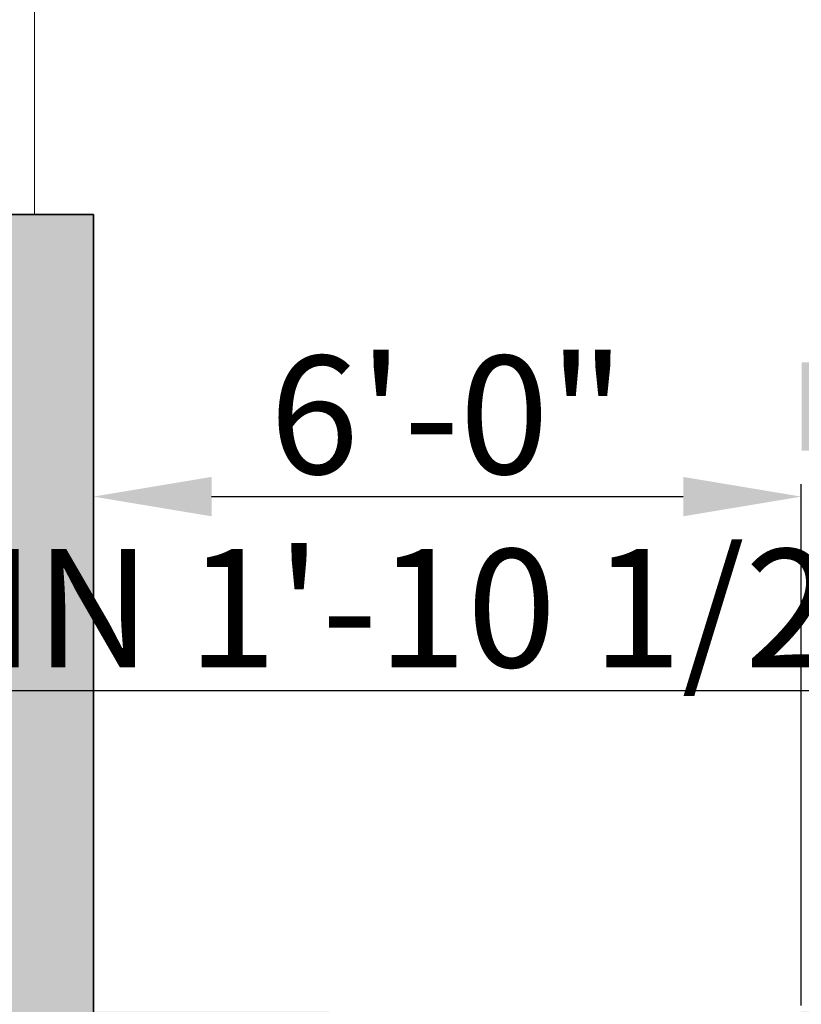
# Model space of a CAD drawing. Units: inches. Extents: x 2083 to 3317, y 1141 to 2115.
# Tile 114 of 256: x 2864 to 2944, y 1422 to 1522. Entities that reach past the tile are written whole.
import ezdxf

# ---------------------------------------------------------------- set-up
doc = ezdxf.new("R2010")
doc.units = ezdxf.units.IN
for name, color, linetype, lineweight in [('A-ANNO-DIMS', 2, 'Continuous', 18), ('A-GLAZ', 4, 'Continuous', 18), ('A-WALL', 7, 'Continuous', 35)]:
    doc.layers.add(name, color=color, linetype=linetype, lineweight=lineweight)
doc.layers.add('A-WALL-PATT', color=251, linetype='Continuous', lineweight=13, true_color=0x636466)
doc.styles.get("Standard").update_dxf_attribs({"font": 'arial.ttf'})
doc.dimstyles.new('ISO-25', dxfattribs={"dimtxt": 12, "dimasz": 12, "dimexe": 1.25, "dimexo": 0.625, "dimtad": 1, "dimlunit": 3, "dimtxsty": 'Standard', "dimcen": 2.5, "dimadec": 0, "dimazin": 0, "dimtfac": 1, "dimtmove": 0, "dimatfit": 3, "dimfxl": 1, "dimarcsym": 0})

# ---------------------------------------------------------------- blocks, each defined once
blk = doc.blocks.new('*D18')
at = {"layer": 'A-ANNO-DIMS', "color": 0, "lineweight": -2, "transparency": 16777216}
for p, q in [((3018.48, 1456.16), (3018.48, 1452.14)), ((3041.07, 1456.16), (3041.07, 1452.14)), ((3006.48, 1453.39), (2828.36, 1453.39)), ((3041.07, 1453.39), (3018.48, 1453.39)), ((3053.07, 1453.39), (3065.07, 1453.39))]:
    blk.add_line(p, q, dxfattribs=at)
at = {"layer": 'A-ANNO-DIMS', "color": 0, "transparency": 16777216}
for points in [[(3006.48, 1455.39), (3006.48, 1451.39), (3018.48, 1453.39)], [(3053.07, 1455.39), (3053.07, 1451.39), (3041.07, 1453.39)]]:
    blk.add_solid(points, dxfattribs=at)
at = {"layer": 'Defpoints', "color": 0, "transparency": 16777216}
for p in [(3018.48, 1456.78), (3041.07, 1456.78), (3018.48, 1453.39)]:
    blk.add_point(p, dxfattribs=at)
at = {"layer": 'A-ANNO-DIMS', "color": 0, "transparency": 16777216, "insert": (2911.42, 1460.22), "char_height": 12, "attachment_point": 5}
blk.add_mtext('BASIN 1\'-10 1/2" TYP.', dxfattribs=at)
blk = doc.blocks.new('*D48')
at = {"layer": 'A-ANNO-DIMS', "color": 0, "lineweight": -2, "transparency": 16777216}
for p, q in [((2871.96, 1421.39), (2871.96, 1474.36)), ((2943.91, 1421.39), (2943.91, 1474.36)), ((2883.96, 1473.11), (2931.91, 1473.11))]:
    blk.add_line(p, q, dxfattribs=at)
at = {"layer": 'A-ANNO-DIMS', "color": 0, "transparency": 16777216}
for points in [[(2883.96, 1475.11), (2883.96, 1471.11), (2871.96, 1473.11)], [(2931.91, 1475.11), (2931.91, 1471.11), (2943.91, 1473.11)]]:
    blk.add_solid(points, dxfattribs=at)
at = {"layer": 'Defpoints', "color": 0, "transparency": 16777216}
for p in [(2943.91, 1473.11), (2871.96, 1420.76), (2943.91, 1420.76)]:
    blk.add_point(p, dxfattribs=at)
at = {"layer": 'A-ANNO-DIMS', "color": 0, "transparency": 16777216, "insert": (2907.93, 1479.86), "char_height": 12, "attachment_point": 5}
blk.add_mtext('6\'-0"', dxfattribs=at)
blk = doc.blocks.new('*D57')
at = {"layer": 'A-ANNO-DIMS', "color": 0, "lineweight": -2, "transparency": 16777216}
for p, q in [((2871.33, 1621.76), (2818.36, 1621.76)), ((2819.61, 1513.76), (2819.61, 1609.76)), ((2871.33, 1501.76), (2818.36, 1501.76))]:
    blk.add_line(p, q, dxfattribs=at)
at = {"layer": 'A-ANNO-DIMS', "color": 0, "transparency": 16777216}
for points in [[(2817.61, 1609.76), (2821.61, 1609.76), (2819.61, 1621.76)], [(2817.61, 1513.76), (2821.61, 1513.76), (2819.61, 1501.76)]]:
    blk.add_solid(points, dxfattribs=at)
at = {"layer": 'Defpoints', "color": 0, "transparency": 16777216}
for p in [(2819.61, 1621.76), (2871.96, 1621.76), (2871.96, 1501.76)]:
    blk.add_point(p, dxfattribs=at)
at = {"layer": 'A-ANNO-DIMS', "color": 0, "transparency": 16777216, "insert": (2812.86, 1561.76), "char_height": 12, "attachment_point": 5, "rotation": 90}
blk.add_mtext('10\'-0"', dxfattribs=at)

msp = doc.modelspace()

# ---------------------------------------------------------------- hatches: boundary and pattern name
at = {"layer": 'A-WALL-PATT'}
h = msp.add_hatch(color=256, dxfattribs=at)
h.dxf.hatch_style = 1
h.paths.add_polyline_path([(3126.96, 2020.761), (2748.96, 2020.761), (2604.96, 2020.761), (2226.96, 2020.761), (2226.96, 1702.761), (2466.96, 1702.761), (2466.96, 1582.761), (2418.96, 1582.761), (2418.96, 1477.761), (2226.96, 1477.761), (2226.96, 1263.261), (2544.96, 1263.261), (2544.96, 1411.761), (2604.96, 1411.761), (2685.96, 1411.761), (2685.96, 1420.761), (2604.96, 1420.761), (2604.96, 1573.761), (2604.96, 1702.761), (2604.96, 2011.761), (2748.96, 2011.761), (2748.96, 1702.761), (2862.96, 1702.761), (2862.96, 1621.761), (2871.96, 1621.761), (2871.96, 1702.761), (2883.96, 1702.761), (2883.96, 1706.939, -0.0264593), (2883.96, 1711.761), (2757.96, 1711.761), (2757.96, 1807.761), (2787.96, 1807.761), (2787.96, 1812.261), (2757.96, 1812.261), (2757.96, 2011.761), (2877.96, 2011.761), (2877.96, 1812.261), (2847.96, 1812.261), (2847.96, 1807.761), (2889.836, 1807.761), (2889.836, 1812.261), (2882.46, 1812.261), (2882.46, 2011.761), (3117.96, 2011.761), (3117.96, 1812.261), (2937.836, 1812.261), (2937.836, 1807.761), (2995.71, 1807.761), (2995.71, 1796.118), (3000.21, 1796.118), (3000.21, 1807.761), (3117.96, 1807.761), (3117.96, 1711.761), (3000.21, 1711.761), (3000.21, 1760.118), (2998.573, 1760.118, -0.020711), (2995.71, 1760.118), (2995.71, 1711.761), (2931.96, 1711.761), (2931.96, 1702.761), (3126.96, 1702.761)])
h.paths.add_polyline_path([(2471.46, 2011.761), (2471.46, 1810.011), (2462.717, 1810.011), (2462.717, 1805.511), (2505.96, 1805.511), (2505.96, 1810.011), (2475.96, 1810.011), (2475.96, 2011.761), (2595.96, 2011.761), (2595.96, 1810.011), (2565.96, 1810.011), (2565.96, 1805.511), (2595.96, 1805.511), (2595.96, 1711.761), (2235.96, 1711.761), (2235.96, 1805.511), (2353.71, 1805.511), (2353.71, 1796.054), (2358.21, 1796.054), (2358.21, 1805.511), (2414.717, 1805.511), (2414.717, 1810.011), (2235.96, 1810.011), (2235.96, 2011.761)], flags=16)
h.paths.add_polyline_path([(2270.205, 1994.61), (2270.205, 1970.61), (2246.205, 1970.61), (2246.205, 1994.61)], flags=0)
edge = h.paths.add_edge_path(flags=0)
edge.add_ellipse((2332.027, 1899.798), major_axis=(-3.043, 3.043), ratio=0.1682525, start_angle=-161.33217, end_angle=-156.30711, ccw=False)
edge.add_ellipse((2333.082, 1898.744), major_axis=(-1.055, 1.055), ratio=0.4535321, start_angle=-123.37102, end_angle=-94.15911)
edge = h.paths.add_edge_path(flags=0)
edge.add_ellipse((2332.027, 1968.876), major_axis=(3.043, 3.043), ratio=0.1682525, start_angle=18.66783, end_angle=23.69289)
edge.add_spline(control_points=[(2332.926, 1970.691), (2332.227, 1970.336), (2330.894, 1969.659), (2328.413, 1970.932), (2327.204, 1967.749), (2324.71, 1969.956), (2322.533, 1967.012), (2320.013, 1971.296), (2317.68, 1968.158), (2316.041, 1967.102), (2315.427, 1966.81)], knot_values=[0, 0, 0, 0, 2.2670587, 4.3245589, 6.6855835, 8.8786411, 11.121502, 14.300359, 17.7552837, 19.732645, 19.732645, 19.732645, 19.732645], degree=3, periodic=0)
edge.add_ellipse((2332.027, 1968.876), major_axis=(3.043, 3.043), ratio=0.1682525, start_angle=18.66783, end_angle=23.69289, ccw=False)
edge.add_ellipse((2333.082, 1969.931), major_axis=(1.055, 1.055), ratio=0.4535321, start_angle=56.62898, end_angle=85.84089, ccw=False)
edge = h.paths.add_edge_path(flags=0)
edge.add_spline(control_points=[(2296.428, 1967.988), (2293.628, 1965.336), (2287.704, 1959.727), (2299.744, 1949.996), (2294.533, 1935.669), (2290.573, 1920.604), (2293.394, 1909.974), (2296.185, 1904.967)], knot_values=[0.0991853, 0.0991853, 0.0991853, 0.0991853, 0.3453009, 0.6198217, 0.9826526, 1.3860932, 1.8105546, 1.8105546, 1.8105546, 1.8105546], degree=3, periodic=0)
edge.add_spline(control_points=[(2296.185, 1904.967), (2297.384, 1902.619), (2298.001, 1901.949), (2298.553, 1901.468)], knot_values=[0.0062457, 0.0062457, 0.0062457, 0.0062457, 0.0554759, 0.0554759, 0.0554759, 0.0554759], degree=3, periodic=0)
edge.add_spline(control_points=[(2298.553, 1901.468), (2297.259, 1900.923), (2295.225, 1900.232), (2293.06, 1900.614), (2292.101, 1900.788), (2292.09, 1900.791)], knot_values=[0.3128349, 0.3128349, 0.3128349, 0.3128349, 0.4017797, 0.4749867, 0.4759027, 0.4759027, 0.4759027, 0.4759027], degree=3, periodic=0)
edge.add_arc((2292.794, 1904.664), 3.937, 215.4209, 259.69818, ccw=False)
edge.add_spline(control_points=[(2289.585, 1902.382), (2289.477, 1902.535), (2289.368, 1902.688), (2289.261, 1902.841)], knot_values=[0.1028719, 0.1028719, 0.1028719, 0.1028719, 0.1168958, 0.1168958, 0.1168958, 0.1168958], degree=3, periodic=0)
edge.add_spline(control_points=[(2289.261, 1902.841), (2288.687, 1902.55), (2287.64, 1902.02), (2285.881, 1901.874), (2283.853, 1901.504), (2281.72, 1899.711), (2278.467, 1899.493), (2276.157, 1901.883), (2272.259, 1899.804), (2267.778, 1901.843), (2262.244, 1900.184), (2257.415, 1901.782), (2254.318, 1900.726), (2253.178, 1900.337)], knot_values=[0, 0, 0, 0, 1.9079767, 3.4771759, 5.261074, 7.9728515, 11.6802485, 13.7179214, 16.9395917, 22.789562, 27.5025027, 33.5952153, 37.1456181, 37.1456181, 37.1456181, 37.1456181], degree=3, periodic=0)
edge.add_line((2253.178, 1900.337), (2250.244, 1902.841))
edge.add_line((2250.244, 1902.841), (2250.244, 1965.833))
edge.add_line((2250.244, 1965.833), (2253.178, 1968.337))
edge.add_spline(control_points=[(2253.178, 1968.337), (2254.318, 1967.948), (2257.415, 1966.892), (2262.244, 1968.49), (2267.778, 1966.831), (2271.527, 1968.537), (2273.876, 1967.828), (2274.207, 1967.728)], knot_values=[0, 0, 0, 0, 0.0901802, 0.2449351, 0.3646438, 0.5132331, 0.5378548, 0.5378548, 0.5378548, 0.5378548], degree=3, periodic=0)
edge.add_arc((2274.353, 1963.793), 3.937, 72.05113, 92.12795, ccw=False)
edge.add_arc((2281.297, 1985.23), 18.596, 252.05113, 288.56572)
edge.add_arc((2292.317, 1956.029), 12.646, 71.02679, 113.77822, ccw=False)
edge = h.paths.add_edge_path(flags=0)
edge.add_spline(control_points=[(2274.899, 1951.856), (2275.066, 1951.617), (2275.233, 1951.377), (2275.398, 1951.136)], knot_values=[1.4099157, 1.4099157, 1.4099157, 1.4099157, 1.4315903, 1.4315903, 1.4315903, 1.4315903], degree=3, periodic=0)
edge.add_spline(control_points=[(2275.398, 1951.136), (2275.792, 1950.562), (2276.179, 1949.984), (2276.546, 1949.397)], knot_values=[1.3582378, 1.3582378, 1.3582378, 1.3582378, 1.4099157, 1.4099157, 1.4099157, 1.4099157], degree=3, periodic=0)
edge.add_line((2276.546, 1949.397), (2277.437, 1947.862))
edge.add_spline(control_points=[(2277.437, 1947.862), (2276.304, 1945.673), (2274.64, 1942.427), (2274.632, 1938.094), (2272.799, 1930.852), (2274.356, 1943.897), (2275.948, 1947.923), (2276.546, 1949.397)], knot_values=[0.0056315, 0.0056315, 0.0056315, 0.0056315, 0.1860139, 0.2660015, 0.3570872, 0.5963902, 0.7397317, 0.7397317, 0.7397317, 0.7397317], degree=3, periodic=0)
edge.add_spline(control_points=[(2276.546, 1949.397), (2276.179, 1949.984), (2275.792, 1950.562), (2275.398, 1951.136)], knot_values=[1.3582378, 1.3582378, 1.3582378, 1.3582378, 1.4099157, 1.4099157, 1.4099157, 1.4099157], degree=3, periodic=0)
edge.add_spline(control_points=[(2275.398, 1951.136), (2274.943, 1950.08), (2274.208, 1948.025), (2273.935, 1944.851), (2272.469, 1937.627), (2273.466, 1945.696), (2274.701, 1951.059), (2274.899, 1951.856)], knot_values=[0.1043639, 0.1043639, 0.1043639, 0.1043639, 0.1896363, 0.2696239, 0.3607096, 0.6000126, 0.6446217, 0.6446217, 0.6446217, 0.6446217], degree=3, periodic=0)
h.paths.add_polyline_path([(2269.168, 1963.128, -0.3575267), (2268.171, 1960.976, -0.0925607), (2268.171, 1939.436, -0.3575267), (2269.168, 1937.285, -0.3575267), (2267.016, 1938.282, -0.1647847), (2254.686, 1938.282, -0.3575267), (2252.534, 1937.285, -0.3575267), (2253.531, 1939.436, -0.0925607), (2253.531, 1960.976, -0.3575267), (2252.534, 1963.128, -0.3575267), (2254.686, 1962.131, -0.1647847), (2267.016, 1962.131, -0.3575267)], flags=0)
h.paths.add_polyline_path([(2248.874, 1967.802), (2248.874, 1957.028), (2249.458, 1957.028), (2249.458, 1911.647), (2248.874, 1911.647), (2248.874, 1900.873), (2246.512, 1900.873, 0.1973271), (2244.15, 1902.457), (2244.15, 1966.218, 0.1973271), (2246.512, 1967.802)], flags=0)
h.paths.add_polyline_path([(2269.168, 1931.389, -0.3575267), (2268.171, 1929.238, -0.0925607), (2268.171, 1907.698, -0.3575267), (2269.168, 1905.547, -0.3575267), (2267.016, 1906.544, -0.1647847), (2254.686, 1906.544, -0.3575267), (2252.534, 1905.547, -0.3575267), (2253.531, 1907.698, -0.0925607), (2253.531, 1929.238, -0.3575267), (2252.534, 1931.389, -0.3575267), (2254.686, 1930.392, -0.1647847), (2267.016, 1930.392, -0.3575267)], flags=0)
edge = h.paths.add_edge_path(flags=0)
edge.add_spline(control_points=[(2276.197, 1906.724), (2276.168, 1909.029), (2276.114, 1913.372), (2270.598, 1924.925), (2273.905, 1919.013), (2275.922, 1916.262), (2275.475, 1912.402), (2277.258, 1910.381), (2276.696, 1908.225), (2276.646, 1906.813), (2276.618, 1906.008)], knot_values=[0, 0, 0, 0, 8.6102597, 16.2212739, 18.8430575, 23.8048978, 27.4408283, 29.3561016, 31.2034776, 33.6506866, 33.6506866, 33.6506866, 33.6506866], degree=3, periodic=0)
edge.add_spline(control_points=[(2276.618, 1906.008), (2276.623, 1905.624), (2276.498, 1904.629), (2275.442, 1903.855), (2274.937, 1903.08), (2274.859, 1902.841)], knot_values=[0.1564884, 0.1564884, 0.1564884, 0.1564884, 0.1843975, 0.2313765, 0.2505985, 0.2505985, 0.2505985, 0.2505985], degree=3, periodic=0)
edge.add_line((2274.859, 1902.841), (2276.506, 1902.841))
edge.add_spline(control_points=[(2276.506, 1902.841), (2276.788, 1903.085), (2277.665, 1904.125), (2278.25, 1904.341), (2277.654, 1908.527), (2278.156, 1906.228), (2278.1, 1905.286), (2278.847, 1904.069), (2277.857, 1903.415), (2277.874, 1902.991), (2277.904, 1902.841)], knot_values=[0.0595743, 0.0595743, 0.0595743, 0.0595743, 0.0807529, 0.1037415, 0.1697201, 0.1760361, 0.2071372, 0.2404744, 0.2623409, 0.2736605, 0.2736605, 0.2736605, 0.2736605], degree=3, periodic=0)
edge.add_line((2277.904, 1902.841), (2280.03, 1902.841))
edge.add_spline(control_points=[(2280.03, 1902.841), (2279.888, 1903.088), (2279.499, 1903.982), (2280.152, 1905.939), (2278.104, 1909.658), (2279.762, 1907.185), (2280.328, 1904.875), (2280.485, 1903.49), (2281.463, 1903.249), (2281.758, 1902.936), (2281.834, 1902.841)], knot_values=[0.013856, 0.013856, 0.013856, 0.013856, 0.0348738, 0.0888667, 0.1078792, 0.1267378, 0.158714, 0.1937575, 0.2174868, 0.2267221, 0.2267221, 0.2267221, 0.2267221], degree=3, periodic=0)
edge.add_spline(control_points=[(2281.834, 1902.841), (2281.788, 1902.827), (2281.647, 1902.783), (2281.396, 1902.859), (2281.088, 1902.985), (2280.721, 1903.061), (2280.333, 1903.026), (2280.125, 1902.899), (2280.03, 1902.841)], knot_values=[0, 0, 0, 0, 0.1441304, 0.435517, 0.7492759, 1.1530457, 1.5483707, 1.878348, 1.878348, 1.878348, 1.878348], degree=3, periodic=0)
edge.add_line((2280.03, 1902.841), (2277.904, 1902.841))
edge.add_spline(control_points=[(2277.904, 1902.841), (2277.893, 1902.796), (2277.865, 1902.68), (2277.607, 1902.687), (2277.274, 1902.801), (2276.838, 1902.62), (2276.584, 1902.789), (2276.506, 1902.841)], knot_values=[0, 0, 0, 0, 0.1271885, 0.3261988, 0.6280094, 1.2435704, 1.5153306, 1.5153306, 1.5153306, 1.5153306], degree=3, periodic=0)
edge.add_line((2276.506, 1902.841), (2274.859, 1902.841))
edge.add_spline(control_points=[(2274.859, 1902.841), (2274.814, 1902.899), (2274.725, 1903.013), (2274.493, 1903.119), (2274.244, 1902.961), (2273.937, 1903.185), (2273.614, 1902.983), (2273.408, 1902.883), (2273.322, 1902.841)], knot_values=[0, 0, 0, 0, 0.2184302, 0.4369566, 0.6879766, 0.9903786, 1.3983955, 1.6918498, 1.6918498, 1.6918498, 1.6918498], degree=3, periodic=0)
edge.add_spline(control_points=[(2273.322, 1902.841), (2273.617, 1903.446), (2274.274, 1904.538), (2276.027, 1904.574), (2276.207, 1906.584), (2276.197, 1906.724)], knot_values=[0.0122268, 0.0122268, 0.0122268, 0.0122268, 0.0594721, 0.1062177, 0.134458, 0.134458, 0.134458, 0.134458], degree=3, periodic=0)
h.paths.add_polyline_path([(2270.776, 1897.79), (2270.776, 1873.79), (2246.776, 1873.79), (2246.776, 1897.79)], flags=0)
h.paths.add_polyline_path([(2353.71, 1760.005), (2353.71, 1760.054), (2358.21, 1760.054, -0.033729)], flags=0)
h.paths.add_polyline_path([(2321.819, 1737.529), (2341.995, 1737.529, -0.4142136), (2343.203, 1736.321), (2343.203, 1721.021, -0.4142136), (2341.995, 1719.813), (2321.819, 1719.813, -0.4142136), (2320.611, 1721.021), (2320.611, 1736.321, -0.4142136)], flags=0)
h.paths.add_polyline_path([(2324.235, 1736.321), (2339.579, 1736.321, -0.4142136), (2341.995, 1733.905), (2341.995, 1725.45, -0.4142136), (2339.579, 1723.034), (2333.681, 1723.034), (2333.845, 1722.045, -0.8706461), (2335.425, 1721.826, -0.767327), (2333.923, 1721.423), (2331.291, 1721.423, -0.767327), (2329.788, 1721.826, -0.8706461), (2331.368, 1722.045), (2331.533, 1723.034), (2324.235, 1723.034, -0.4142136), (2321.819, 1725.45), (2321.819, 1733.905, -0.4142136)], flags=0)
h.paths.add_polyline_path([(2570.484, 1928.615), (2589.684, 1928.615), (2590.169, 1928.615), (2590.169, 1904.993), (2570.484, 1904.993)], flags=0)
h.paths.add_polyline_path([(2574.447, 1927.264, -1), (2572.829, 1927.264, -1)], flags=0)
h.paths.add_polyline_path([(2573.09, 1926.941), (2573.925, 1927.776), (2574.148, 1927.553), (2573.313, 1926.718)], flags=0)
h.paths.add_polyline_path([(2578.779, 1919.73, -1), (2571.592, 1919.73, -1)], flags=0)
h.paths.add_polyline_path([(2578.385, 1919.73, -1), (2571.985, 1919.73, -1)], flags=0)
h.paths.add_polyline_path([(2331.596, 1729.476, -1), (2333.618, 1729.476, -1)], flags=0)
h.paths.add_polyline_path([(2578.034, 1927.264, -1), (2576.416, 1927.264, -1)], flags=0)
h.paths.add_polyline_path([(2576.689, 1927.531), (2576.912, 1927.754), (2577.747, 1926.919), (2577.524, 1926.696)], flags=0)
h.paths.add_polyline_path([(2578.139, 1909.86, -1), (2572.232, 1909.86, -1)], flags=0)
h.paths.add_polyline_path([(2577.745, 1909.86, -1), (2572.625, 1909.86, -1)], flags=0)
h.paths.add_polyline_path([(2583.798, 1927.264, -1), (2582.179, 1927.264, -1)], flags=0)
h.paths.add_polyline_path([(2582.719, 1927.754), (2583.554, 1926.919), (2583.331, 1926.696), (2582.496, 1927.531)], flags=0)
h.paths.add_polyline_path([(2582.496, 1927.531), (2582.719, 1927.754), (2583.554, 1926.919), (2583.331, 1926.696)], flags=0)
h.paths.add_polyline_path([(2587.739, 1920.53, -1), (2581.832, 1920.53, -1)], flags=0)
h.paths.add_polyline_path([(2587.345, 1920.53, -1), (2582.225, 1920.53, -1)], flags=0)
h.paths.add_polyline_path([(2587.385, 1927.264, -1), (2585.766, 1927.264, -1)], flags=0)
h.paths.add_polyline_path([(2586.082, 1926.98), (2586.917, 1927.815), (2587.14, 1927.593), (2586.305, 1926.758)], flags=0)
h.paths.add_polyline_path([(2588.379, 1910.66, -1), (2581.192, 1910.66, -1)], flags=0)
h.paths.add_polyline_path([(2587.985, 1910.66, -1), (2581.585, 1910.66, -1)], flags=0)
h.paths.add_polyline_path([(2417.168, 1729.478), (2437.344, 1729.478, -0.4142136), (2438.552, 1728.27), (2438.552, 1712.969, -0.4142136), (2437.344, 1711.761), (2417.168, 1711.761, -0.4142136), (2415.96, 1712.969), (2415.96, 1728.27, -0.4142136)], flags=0)
h.paths.add_polyline_path([(2419.584, 1728.27), (2434.928, 1728.27, -0.4142136), (2437.344, 1725.854), (2437.344, 1717.398, -0.4142136), (2434.928, 1714.983), (2429.029, 1714.983), (2429.194, 1713.994, -0.8706461), (2430.774, 1713.775, -0.767327), (2429.271, 1713.372), (2426.64, 1713.372, -0.767327), (2425.137, 1713.775, -0.8706461), (2426.717, 1713.994), (2426.882, 1714.983), (2419.584, 1714.983, -0.4142136), (2417.168, 1717.398), (2417.168, 1725.854, -0.4142136)], flags=0)
h.paths.add_polyline_path([(2419.584, 1728.27), (2434.928, 1728.27, -0.4142136), (2437.344, 1725.854), (2437.344, 1717.398, -0.4142136), (2434.928, 1714.983), (2429.029, 1714.983), (2428.358, 1719.009), (2427.553, 1719.009), (2426.882, 1714.983), (2419.584, 1714.983, -0.4142136), (2417.168, 1717.398), (2417.168, 1725.854, -0.4142136)], flags=0)
h.paths.add_polyline_path([(2426.944, 1721.425, -1), (2428.967, 1721.425, -1)], flags=0)
h.paths.add_polyline_path([(2475.96, 1702.761), (2595.96, 1702.761), (2595.96, 1582.761), (2475.96, 1582.761)], flags=16)
h.paths.add_polyline_path([(2427.96, 1573.761), (2595.96, 1573.761), (2595.96, 1468.761), (2595.96, 1420.761), (2384.46, 1420.761), (2384.46, 1468.761), (2427.96, 1468.761)], flags=16)
h.paths.add_polyline_path([(2379.96, 1468.761), (2379.96, 1420.761), (2235.96, 1420.761), (2235.96, 1468.761)], flags=16)
h.paths.add_polyline_path([(2317.816, 1466.696), (2337.992, 1466.696, -0.4142136), (2339.2, 1465.488), (2339.2, 1450.187, -0.4142136), (2337.992, 1448.979), (2317.816, 1448.979, -0.4142136), (2316.608, 1450.187), (2316.608, 1465.488, -0.4142136)], flags=0)
h.paths.add_polyline_path([(2320.232, 1465.488), (2335.576, 1465.488, -0.4142136), (2337.992, 1463.072), (2337.992, 1454.616, -0.4142136), (2335.576, 1452.2), (2329.677, 1452.2), (2329.842, 1451.212, -0.8706461), (2331.422, 1450.992, -0.767327), (2329.92, 1450.59), (2327.288, 1450.59, -0.767327), (2325.785, 1450.992, -0.8706461), (2327.365, 1451.212), (2327.53, 1452.2), (2320.232, 1452.2, -0.4142136), (2317.816, 1454.616), (2317.816, 1463.072, -0.4142136)], flags=0)
h.paths.add_polyline_path([(2320.232, 1465.488), (2335.576, 1465.488, -0.4142136), (2337.992, 1463.072), (2337.992, 1454.616, -0.4142136), (2335.576, 1452.2), (2329.677, 1452.2), (2329.006, 1456.227), (2328.201, 1456.227), (2327.53, 1452.2), (2320.232, 1452.2, -0.4142136), (2317.816, 1454.616), (2317.816, 1463.072, -0.4142136)], flags=0)
h.paths.add_polyline_path([(2327.593, 1458.643, -1), (2329.615, 1458.643, -1)], flags=0)
h.paths.add_polyline_path([(2244.412, 1433.34), (2241.921, 1433.34, -0.4142136), (2240.018, 1435.244), (2240.018, 1440.953, -0.4142105), (2241.921, 1442.856), (2244.412, 1442.856, -1.9764724)], flags=0)
h.paths.add_polyline_path([(2245.357, 1434.398, -0.4142136), (2245.357, 1441.799, -2.1440985)], flags=0)
h.paths.add_polyline_path([(2535.96, 1416.261), (2535.96, 1272.261), (2235.96, 1272.261), (2235.96, 1416.261)], flags=16)
h.paths.add_polyline_path([(2260.12, 1384.293), (2260.12, 1362.039), (2237.865, 1362.039), (2237.865, 1384.293)], flags=0)
edge = h.paths.add_edge_path(flags=0)
edge.add_line((2318.252, 1362.093), (2318.146, 1362.001))
edge.add_ellipse((2317.445, 1360.431), major_axis=(2.822, 2.822), ratio=0.1682525, start_angle=18.66783, end_angle=20.94813, ccw=False)
edge.add_ellipse((2318.423, 1361.409), major_axis=(0.978, 0.978), ratio=0.4535321, start_angle=56.62898, end_angle=70.2262, ccw=False)
edge = h.paths.add_edge_path(flags=0)
edge.add_line((2319.107, 1295.571), (2319.015, 1295.677))
edge.add_ellipse((2317.445, 1296.378), major_axis=(-2.822, 2.822), ratio=0.1682525, start_angle=-161.33217, end_angle=-159.05187, ccw=False)
edge.add_ellipse((2318.423, 1295.4), major_axis=(-0.978, 0.978), ratio=0.4535321, start_angle=-123.37102, end_angle=-109.7738)
edge = h.paths.add_edge_path(flags=0)
edge.add_spline(control_points=[(2284.21, 1301.17), (2284.581, 1300.445), (2284.891, 1299.892), (2285.16, 1299.461)], knot_values=[0.0390658, 0.0390658, 0.0390658, 0.0390658, 0.0554759, 0.0554759, 0.0554759, 0.0554759], degree=3, periodic=0)
edge.add_line((2285.16, 1299.461), (2284.21, 1301.17))
edge = h.paths.add_edge_path(flags=0)
edge.add_line((2280.412, 1297.298), (2283.37, 1297.036))
edge.add_line((2283.37, 1297.036), (2286.406, 1297.926))
edge.add_spline(control_points=[(2286.406, 1297.926), (2285.305, 1297.463), (2284.345, 1297.129), (2283.37, 1297.036)], knot_values=[0.3943688, 0.3943688, 0.3943688, 0.3943688, 0.4759027, 0.4759027, 0.4759027, 0.4759027], degree=3, periodic=0)
edge.add_spline(control_points=[(2283.37, 1297.036), (2283.281, 1297.028), (2282.316, 1296.957), (2281.313, 1297.134), (2280.423, 1297.296), (2280.412, 1297.298)], knot_values=[0.3128349, 0.3128349, 0.3128349, 0.3128349, 0.3202458, 0.3934528, 0.3943688, 0.3943688, 0.3943688, 0.3943688], degree=3, periodic=0)
edge = h.paths.add_edge_path(flags=0)
edge.add_line((2284.436, 1359.607), (2280.446, 1355.328))
edge.add_line((2280.446, 1355.328), (2279.58, 1351.018))
edge.add_line((2279.58, 1351.018), (2282.413, 1346.58))
edge.add_spline(control_points=[(2282.413, 1346.58), (2283.153, 1345.589), (2284.253, 1344.029), (2284.801, 1342.387), (2284.935, 1341.806)], knot_values=[1.2400982, 1.2400982, 1.2400982, 1.2400982, 1.3328922, 1.3827123, 1.3827123, 1.3827123, 1.3827123], degree=3, periodic=0)
edge.add_spline(control_points=[(2284.935, 1341.806), (2285.319, 1340.141), (2285.233, 1338.409), (2284.91, 1336.654)], knot_values=[1.0974841, 1.0974841, 1.0974841, 1.0974841, 1.2400982, 1.2400982, 1.2400982, 1.2400982], degree=3, periodic=0)
edge.add_spline(control_points=[(2284.91, 1336.654), (2284.587, 1334.899), (2284.027, 1333.12), (2283.463, 1331.361)], knot_values=[0.9548699, 0.9548699, 0.9548699, 0.9548699, 1.0974841, 1.0974841, 1.0974841, 1.0974841], degree=3, periodic=0)
edge.add_line((2283.463, 1331.361), (2281.89, 1326.153))
edge.add_line((2281.89, 1326.153), (2280.756, 1321.056))
edge.add_line((2280.756, 1321.056), (2280.299, 1316.002))
edge.add_line((2280.299, 1316.002), (2280.716, 1310.95))
edge.add_line((2280.716, 1310.95), (2282.028, 1305.972))
edge.add_line((2282.028, 1305.972), (2284.21, 1301.17))
edge.add_spline(control_points=[(2284.21, 1301.17), (2283.341, 1302.73), (2282.612, 1304.336), (2282.028, 1305.972)], knot_values=[0.0991853, 0.0991853, 0.0991853, 0.0991853, 0.2417994, 0.2417994, 0.2417994, 0.2417994], degree=3, periodic=0)
edge.add_spline(control_points=[(2282.028, 1305.972), (2281.444, 1307.608), (2281.005, 1309.273), (2280.716, 1310.95)], knot_values=[0.2417994, 0.2417994, 0.2417994, 0.2417994, 0.3844135, 0.3844135, 0.3844135, 0.3844135], degree=3, periodic=0)
edge.add_spline(control_points=[(2280.716, 1310.95), (2280.433, 1312.588), (2280.289, 1314.277), (2280.299, 1315.962), (2280.299, 1316.002)], knot_values=[0.3844135, 0.3844135, 0.3844135, 0.3844135, 0.5236467, 0.5270276, 0.5270276, 0.5270276, 0.5270276], degree=3, periodic=0)
edge.add_spline(control_points=[(2280.299, 1316.002), (2280.312, 1317.687), (2280.478, 1319.368), (2280.756, 1321.056)], knot_values=[0.5270276, 0.5270276, 0.5270276, 0.5270276, 0.6696417, 0.6696417, 0.6696417, 0.6696417], degree=3, periodic=0)
edge.add_spline(control_points=[(2280.756, 1321.056), (2281.035, 1322.744), (2281.426, 1324.44), (2281.89, 1326.153)], knot_values=[0.6696417, 0.6696417, 0.6696417, 0.6696417, 0.8122558, 0.8122558, 0.8122558, 0.8122558], degree=3, periodic=0)
edge.add_spline(control_points=[(2281.89, 1326.153), (2282.264, 1327.533), (2282.788, 1329.262), (2283.353, 1331.018), (2283.463, 1331.361)], knot_values=[0.8122558, 0.8122558, 0.8122558, 0.8122558, 0.9270873, 0.9548699, 0.9548699, 0.9548699, 0.9548699], degree=3, periodic=0)
edge.add_line((2283.463, 1331.361), (2284.91, 1336.654))
edge.add_line((2284.91, 1336.654), (2284.935, 1341.806))
edge.add_line((2284.935, 1341.806), (2282.413, 1346.58))
edge.add_spline(control_points=[(2282.413, 1346.58), (2281.275, 1348.104), (2280.078, 1349.57), (2279.58, 1351.018)], knot_values=[1.3827123, 1.3827123, 1.3827123, 1.3827123, 1.5253264, 1.5253264, 1.5253264, 1.5253264], degree=3, periodic=0)
edge.add_spline(control_points=[(2279.58, 1351.018), (2279.443, 1351.415), (2279.136, 1352.857), (2279.735, 1354.29), (2280.446, 1355.328)], knot_values=[1.5253264, 1.5253264, 1.5253264, 1.5253264, 1.564439, 1.6679405, 1.6679405, 1.6679405, 1.6679405], degree=3, periodic=0)
edge.add_spline(control_points=[(2280.446, 1355.328), (2281.426, 1356.758), (2282.931, 1358.183), (2284.436, 1359.607)], knot_values=[1.6679405, 1.6679405, 1.6679405, 1.6679405, 1.8105546, 1.8105546, 1.8105546, 1.8105546], degree=3, periodic=0)
edge.add_arc((2280.623, 1348.518), 11.726, 71.02679, 113.77822)
edge.add_arc((2270.405, 1375.595), 17.244, 252.05113, 288.56572, ccw=False)
edge.add_arc((2263.966, 1355.718), 3.651, 72.05113, 92.12795)
edge.add_arc((2263.966, 1355.718), 3.651, 92.12795, 177.98513)
edge.add_spline(control_points=[(2260.318, 1355.846), (2260.26, 1354.221), (2260.551, 1350.187), (2262.999, 1346.766), (2264.473, 1344.649)], knot_values=[1.4315903, 1.4315903, 1.4315903, 1.4315903, 1.5641438, 1.7706953, 1.7706953, 1.7706953, 1.7706953], degree=3, periodic=0)
edge.add_line((2264.473, 1344.649), (2264.936, 1343.983))
edge.add_spline(control_points=[(2263.801, 1340.248), (2263.843, 1340.514), (2264.067, 1341.756), (2264.513, 1343.002), (2264.935, 1343.981)], knot_values=[0.5365702, 0.5365702, 0.5365702, 0.5365702, 0.5593494, 0.6446217, 0.6446217, 0.6446217, 0.6446217], degree=3, periodic=0)
edge.add_spline(control_points=[(2264.935, 1343.981), (2265.118, 1343.715), (2265.299, 1343.448), (2265.477, 1343.179)], knot_values=[1.3840767, 1.3840767, 1.3840767, 1.3840767, 1.4099157, 1.4099157, 1.4099157, 1.4099157], degree=3, periodic=0)
edge.add_spline(control_points=[(2265.477, 1343.179), (2265.655, 1342.911), (2265.829, 1342.641), (2265.999, 1342.369)], knot_values=[1.3582378, 1.3582378, 1.3582378, 1.3582378, 1.3840767, 1.3840767, 1.3840767, 1.3840767], degree=3, periodic=0)
edge.add_line((2265.999, 1342.369), (2266.826, 1340.946))
edge.add_spline(control_points=[(2266.826, 1340.946), (2268.894, 1337.09), (2271.398, 1325.843), (2270.516, 1310.569), (2275.919, 1301.861), (2277.79, 1299.199)], knot_values=[0.1168958, 0.1168958, 0.1168958, 0.1168958, 0.4729873, 1.0509689, 1.3137934, 1.3137934, 1.3137934, 1.3137934], degree=3, periodic=0)
edge.add_spline(control_points=[(2277.79, 1299.199), (2277.839, 1299.128), (2277.889, 1299.057), (2277.94, 1298.987)], knot_values=[0.1098839, 0.1098839, 0.1098839, 0.1098839, 0.1168958, 0.1168958, 0.1168958, 0.1168958], degree=3, periodic=0)
edge.add_line((2277.94, 1298.987), (2277.789, 1299.199))
edge.add_spline(control_points=[(2277.789, 1299.199), (2277.257, 1298.929), (2276.286, 1298.438), (2275.039, 1298.334), (2274.383, 1298.239), (2274.215, 1298.209)], knot_values=[33.1218702, 33.1218702, 33.1218702, 33.1218702, 35.0290557, 36.5982549, 37.1448269, 37.1448269, 37.1448269, 37.1448269], degree=3, periodic=0)
edge.add_line((2274.215, 1298.209), (2273.073, 1297.893))
edge.add_spline(control_points=[(2273.073, 1297.893), (2272.323, 1297.58), (2271.039, 1296.511), (2269.248, 1296.226), (2268.423, 1296.375)], knot_values=[26.5325843, 26.5325843, 26.5325843, 26.5325843, 29.198919, 31.8391012, 31.8391012, 31.8391012, 31.8391012], degree=3, periodic=0)
edge.add_line((2268.423, 1296.375), (2263.879, 1297.458))
edge.add_spline(control_points=[(2263.879, 1297.458), (2263.556, 1297.359), (2261.86, 1296.839), (2260.239, 1297.282), (2258.933, 1297.516)], knot_values=[15.9195506, 15.9195506, 15.9195506, 15.9195506, 16.9395917, 21.2260675, 21.2260675, 21.2260675, 21.2260675], degree=3, periodic=0)
edge.add_line((2258.933, 1297.516), (2254.055, 1297.329))
edge.add_spline(control_points=[(2254.055, 1297.329), (2253.756, 1297.296), (2252.114, 1297.165), (2250.462, 1297.544), (2249.13, 1297.668)], knot_values=[5.3065169, 5.3065169, 5.3065169, 5.3065169, 6.2764352, 10.6130337, 10.6130337, 10.6130337, 10.6130337], degree=3, periodic=0)
edge.add_line((2249.13, 1297.668), (2244.332, 1296.878))
edge.add_line((2244.332, 1296.878), (2241.611, 1299.199))
edge.add_line((2241.611, 1299.199), (2241.611, 1357.609))
edge.add_line((2241.611, 1357.609), (2244.332, 1359.931))
edge.add_line((2244.332, 1359.931), (2252.729, 1359.543))
edge.add_spline(control_points=[(2252.729, 1359.543), (2252.871, 1359.546), (2253.306, 1359.548), (2253.74, 1359.514), (2254.032, 1359.482)], knot_values=[0.233291, 0.233291, 0.233291, 0.233291, 0.2449351, 0.2689274, 0.2689274, 0.2689274, 0.2689274], degree=3, periodic=0)
edge.add_line((2254.032, 1359.482), (2259.587, 1359.416))
edge.add_spline(control_points=[(2259.587, 1359.416), (2260.677, 1359.629), (2262.073, 1359.897), (2263.524, 1359.459), (2263.83, 1359.366)], knot_values=[0.4225164, 0.4225164, 0.4225164, 0.4225164, 0.5132331, 0.5378548, 0.5378548, 0.5378548, 0.5378548], degree=3, periodic=0)
edge.add_arc((2263.966, 1355.718), 3.651, 72.05113, 92.12795, ccw=False)
edge.add_arc((2270.405, 1375.595), 17.244, 252.05113, 288.56572)
edge.add_arc((2280.623, 1348.518), 11.726, 71.02679, 113.77822, ccw=False)
h.paths.add_polyline_path([(2240.341, 1359.435), (2240.341, 1349.444), (2240.882, 1349.444), (2240.882, 1307.365), (2240.341, 1307.365), (2240.341, 1297.374), (2238.15, 1297.374, 0.1973271), (2235.96, 1298.843), (2235.96, 1357.966, 0.1973271), (2238.15, 1359.435)], flags=0)
h.paths.add_polyline_path([(2259.158, 1355.101, -0.3575267), (2258.233, 1353.106, -0.0925607), (2258.233, 1333.133, -0.3575267), (2259.158, 1331.138, -0.3575267), (2257.163, 1332.062, -0.1647847), (2245.729, 1332.062, -0.3575267), (2243.735, 1331.138, -0.3575267), (2244.659, 1333.133, -0.0925607), (2244.659, 1353.106, -0.3575267), (2243.735, 1355.101, -0.3575267), (2245.729, 1354.176, -0.1647847), (2257.163, 1354.176, -0.3575267)], flags=0)
edge = h.paths.add_edge_path(flags=0)
edge.add_line((2265.999, 1342.369), (2266.826, 1340.946))
edge.add_line((2266.826, 1340.946), (2265.308, 1337.814))
edge.add_line((2265.308, 1337.814), (2264.358, 1334.653))
edge.add_line((2264.358, 1334.653), (2264.262, 1333.8))
edge.add_spline(control_points=[(2264.262, 1333.8), (2264.208, 1333.187), (2264.162, 1332.366), (2264.007, 1331.414), (2263.969, 1331.202)], knot_values=[0.4644442, 0.4644442, 0.4644442, 0.4644442, 0.5166905, 0.5316081, 0.5316081, 0.5316081, 0.5316081], degree=3, periodic=0)
edge.add_spline(control_points=[(2263.969, 1331.202), (2263.775, 1330.119), (2263.424, 1328.791), (2263.257, 1328.531), (2263.234, 1328.515)], knot_values=[0.3726816, 0.3726816, 0.3726816, 0.3726816, 0.4488497, 0.4644442, 0.4644442, 0.4644442, 0.4644442], degree=3, periodic=0)
edge.add_spline(control_points=[(2263.234, 1328.515), (2263.096, 1328.42), (2263.131, 1329.301), (2263.275, 1330.616)], knot_values=[0.2809191, 0.2809191, 0.2809191, 0.2809191, 0.3726816, 0.3726816, 0.3726816, 0.3726816], degree=3, periodic=0)
edge.add_spline(control_points=[(2263.275, 1330.616), (2263.419, 1331.93), (2263.672, 1333.677), (2263.97, 1335.315)], knot_values=[0.1891566, 0.1891566, 0.1891566, 0.1891566, 0.2809191, 0.2809191, 0.2809191, 0.2809191], degree=3, periodic=0)
edge.add_spline(control_points=[(2263.97, 1335.315), (2264.1, 1336.032), (2264.419, 1337.622), (2264.755, 1338.864), (2264.947, 1339.491)], knot_values=[0.097394, 0.097394, 0.097394, 0.097394, 0.1375775, 0.1891566, 0.1891566, 0.1891566, 0.1891566], degree=3, periodic=0)
edge.add_spline(control_points=[(2264.947, 1339.491), (2265.29, 1340.606), (2265.644, 1341.494), (2265.999, 1342.369)], knot_values=[0.0056315, 0.0056315, 0.0056315, 0.0056315, 0.097394, 0.097394, 0.097394, 0.097394], degree=3, periodic=0)
h.paths.add_polyline_path([(2259.158, 1325.671, -0.3575267), (2258.233, 1323.676, -0.0925607), (2258.233, 1303.703, -0.3575267), (2259.158, 1301.708, -0.3575267), (2257.163, 1302.633, -0.1647847), (2245.729, 1302.633, -0.3575267), (2243.735, 1301.708, -0.3575267), (2244.659, 1303.703, -0.0925607), (2244.659, 1323.676, -0.3575267), (2243.735, 1325.671, -0.3575267), (2245.729, 1324.747, -0.1647847), (2257.163, 1324.747, -0.3575267)], flags=0)
edge = h.paths.add_edge_path(flags=0)
edge.add_spline(control_points=[(2261.709, 1317.311), (2261.679, 1317.418), (2261.762, 1317.389), (2262.491, 1316.09), (2262.962, 1315.301)], knot_values=[14.9558607, 14.9558607, 14.9558607, 14.9558607, 16.2212739, 18.6948259, 18.6948259, 18.6948259, 18.6948259], degree=3, periodic=0)
edge.add_spline(control_points=[(2262.962, 1315.301), (2262.99, 1315.254), (2263.702, 1314.067), (2264.349, 1313.127), (2264.73, 1312.164)], knot_values=[18.6948259, 18.6948259, 18.6948259, 18.6948259, 18.8430575, 22.433791, 22.433791, 22.433791, 22.433791], degree=3, periodic=0)
edge.add_spline(control_points=[(2264.73, 1312.164), (2264.876, 1311.796), (2265.177, 1310.77), (2265.143, 1309.559), (2265.248, 1308.824)], knot_values=[22.433791, 22.433791, 22.433791, 22.433791, 23.8048978, 26.1727562, 26.1727562, 26.1727562, 26.1727562], degree=3, periodic=0)
edge.add_line((2265.248, 1308.824), (2265.851, 1307.172))
edge.add_spline(control_points=[(2265.851, 1307.172), (2266.065, 1306.822), (2266.384, 1306.332), (2266.424, 1305.781), (2266.42, 1305.611)], knot_values=[28.0625624, 28.0625624, 28.0625624, 28.0625624, 29.3561016, 29.9117214, 29.9117214, 29.9117214, 29.9117214], degree=3, periodic=0)
edge.add_spline(control_points=[(2266.42, 1305.611), (2266.416, 1305.433), (2266.394, 1305.25), (2266.365, 1305.066)], knot_values=[29.9117214, 29.9117214, 29.9117214, 29.9117214, 30.4978371, 30.4978371, 30.4978371, 30.4978371], degree=3, periodic=0)
edge.add_line((2266.365, 1305.066), (2266.066, 1302.136))
edge.add_spline(control_points=[(2266.066, 1302.136), (2266.071, 1301.78), (2265.998, 1301.2), (2265.663, 1300.759), (2265.509, 1300.586)], knot_values=[0.1564884, 0.1564884, 0.1564884, 0.1564884, 0.1843975, 0.2035434, 0.2035434, 0.2035434, 0.2035434], degree=3, periodic=0)
edge.add_line((2265.509, 1300.586), (2264.435, 1299.199))
edge.add_line((2264.435, 1299.199), (2265.962, 1299.199))
edge.add_line((2265.962, 1299.199), (2267.336, 1301.175))
edge.add_line((2267.336, 1301.175), (2267.312, 1301.986))
edge.add_spline(control_points=[(2267.312, 1301.986), (2267.261, 1302.862), (2267.16, 1303.737), (2267.271, 1303.326)], knot_values=[0.1262286, 0.1262286, 0.1262286, 0.1262286, 0.1666174, 0.1666174, 0.1666174, 0.1666174], degree=3, periodic=0)
edge.add_spline(control_points=[(2267.271, 1303.326), (2267.28, 1303.294), (2267.31, 1303.175), (2267.373, 1302.884), (2267.406, 1302.683), (2267.418, 1302.601)], knot_values=[0.1666174, 0.1666174, 0.1666174, 0.1666174, 0.1697201, 0.1760361, 0.1807647, 0.1807647, 0.1807647, 0.1807647], degree=3, periodic=0)
edge.add_spline(control_points=[(2267.744, 1300.988), (2267.688, 1301.151), (2267.481, 1301.657), (2267.484, 1302.145), (2267.418, 1302.601)], knot_values=[0.1807647, 0.1807647, 0.1807647, 0.1807647, 0.1937665, 0.2201389, 0.2201389, 0.2201389, 0.2201389], degree=3, periodic=0)
edge.add_line((2267.418, 1302.601), (2267.744, 1300.988))
edge.add_spline(control_points=[(2267.744, 1300.988), (2267.832, 1300.732), (2267.932, 1300.31), (2267.555, 1299.975), (2267.429, 1299.829)], knot_values=[0.2201389, 0.2201389, 0.2201389, 0.2201389, 0.2404744, 0.2548903, 0.2548903, 0.2548903, 0.2548903], degree=3, periodic=0)
edge.add_line((2267.429, 1299.829), (2267.258, 1299.199))
edge.add_line((2267.258, 1299.199), (2269.23, 1299.199))
edge.add_spline(control_points=[(2269.23, 1299.199), (2269.099, 1299.429), (2268.843, 1300.016), (2269.012, 1300.916), (2268.947, 1301.661)], knot_values=[0.013856, 0.013856, 0.013856, 0.013856, 0.0348738, 0.0670726, 0.0670726, 0.0670726, 0.0670726], degree=3, periodic=0)
edge.add_line((2268.947, 1301.661), (2268.432, 1303.603))
edge.add_spline(control_points=[(2268.432, 1303.603), (2268.176, 1304.192), (2267.596, 1305.251), (2268.041, 1304.623), (2268.251, 1304.282)], knot_values=[0.0901547, 0.0901547, 0.0901547, 0.0901547, 0.1078792, 0.1202891, 0.1202891, 0.1202891, 0.1202891], degree=3, periodic=0)
edge.add_spline(control_points=[(2268.251, 1304.282), (2268.361, 1304.105), (2269.058, 1302.918), (2269.383, 1301.59), (2269.521, 1300.776), (2269.575, 1300.556)], knot_values=[0.1202891, 0.1202891, 0.1202891, 0.1202891, 0.1267378, 0.158714, 0.1735056, 0.1735056, 0.1735056, 0.1735056], degree=3, periodic=0)
edge.add_line((2269.575, 1300.556), (2270.686, 1299.421))
edge.add_spline(control_points=[(2270.686, 1299.421), (2270.767, 1299.357), (2270.838, 1299.281), (2270.903, 1299.199)], knot_values=[0.2181597, 0.2181597, 0.2181597, 0.2181597, 0.2267221, 0.2267221, 0.2267221, 0.2267221], degree=3, periodic=0)
edge.add_line((2270.937, 1299.193), (2270.903, 1299.199))
edge.add_spline(control_points=[(2270.903, 1299.199), (2270.86, 1299.186), (2270.73, 1299.146), (2270.496, 1299.216), (2270.272, 1299.308), (2270.121, 1299.348), (2270.063, 1299.36)], knot_values=[0.939174, 0.939174, 0.939174, 0.939174, 1.0833044, 1.3746911, 1.6884499, 1.878348, 1.878348, 1.878348, 1.878348], degree=3, periodic=0)
edge.add_line((2270.063, 1299.36), (2269.23, 1299.199))
edge.add_line((2269.23, 1299.199), (2267.258, 1299.199))
edge.add_spline(control_points=[(2267.258, 1299.199), (2267.248, 1299.157), (2267.223, 1299.05), (2266.984, 1299.057), (2266.809, 1299.116), (2266.677, 1299.109), (2266.637, 1299.105)], knot_values=[0.7576653, 0.7576653, 0.7576653, 0.7576653, 0.8848538, 1.0838641, 1.3856747, 1.5153306, 1.5153306, 1.5153306, 1.5153306], degree=3, periodic=0)
edge.add_spline(control_points=[(2266.637, 1299.105), (2266.485, 1299.089), (2266.236, 1299.017), (2266.035, 1299.151), (2265.962, 1299.199)], knot_values=[0, 0, 0, 0, 0.4859051, 0.7576653, 0.7576653, 0.7576653, 0.7576653], degree=3, periodic=0)
edge.add_line((2265.962, 1299.199), (2264.435, 1299.199))
edge.add_line((2264.435, 1299.199), (2263.858, 1299.367))
edge.add_spline(control_points=[(2263.858, 1299.367), (2263.819, 1299.371), (2263.78, 1299.386), (2263.74, 1299.402)], knot_values=[0.8459249, 0.8459249, 0.8459249, 0.8459249, 0.9786272, 0.9786272, 0.9786272, 0.9786272], degree=3, periodic=0)
edge.add_line((2263.722, 1299.396), (2263.01, 1299.199))
edge.add_spline(control_points=[(2263.01, 1299.199), (2263.246, 1299.683), (2263.506, 1300.128), (2263.873, 1300.408)], knot_values=[0.0122268, 0.0122268, 0.0122268, 0.0122268, 0.0529705, 0.0529705, 0.0529705, 0.0529705], degree=3, periodic=0)
edge.add_spline(control_points=[(2263.873, 1300.408), (2263.932, 1300.453), (2264.084, 1300.553), (2264.255, 1300.624), (2264.36, 1300.665)], knot_values=[0.0529705, 0.0529705, 0.0529705, 0.0529705, 0.0594721, 0.0690861, 0.0690861, 0.0690861, 0.0690861], degree=3, periodic=0)
edge.add_line((2264.36, 1300.665), (2265.142, 1301.078))
edge.add_line((2265.142, 1301.078), (2265.676, 1302.8))
edge.add_line((2265.676, 1302.8), (2265.541, 1305.704))
edge.add_line((2265.541, 1305.704), (2264.803, 1309.328))
edge.add_line((2264.803, 1309.328), (2263.041, 1314.092))
edge.add_spline(control_points=[(2263.041, 1314.092), (2262.384, 1315.671), (2261.796, 1316.998), (2261.709, 1317.311)], knot_values=[11.2168955, 11.2168955, 11.2168955, 11.2168955, 14.9558607, 14.9558607, 14.9558607, 14.9558607], degree=3, periodic=0)
h.paths.add_polyline_path([(2871.96, 1416.261), (2895.91, 1416.261), (2895.91, 1420.761), (2871.96, 1420.761), (2871.96, 1501.761), (2862.96, 1501.761), (2862.96, 1420.761), (2805.96, 1420.761), (2805.96, 1411.761), (2862.96, 1411.761), (2862.96, 1263.261), (3126.96, 1263.261), (3126.96, 1411.761), (3126.96, 1486.761), (2943.96, 1486.761), (2943.96, 1477.761), (2967.86, 1477.761), (2967.86, 1420.761), (2943.91, 1420.761), (2943.91, 1416.261), (3117.96, 1416.261), (3117.96, 1420.761), (2972.36, 1420.761), (2972.36, 1477.761), (3117.96, 1477.761), (3117.96, 1420.761), (3117.96, 1272.261), (2871.96, 1272.261)], flags=0)
h.paths.add_polyline_path([(2457.126, 1485.943), (2527.603, 1485.943), (2527.603, 1537.636), (2457.126, 1537.636)], flags=8)
h.paths.add_polyline_path([(2481.005, 1609.982), (2590.766, 1609.982), (2590.766, 1682.003), (2481.005, 1682.003)], flags=8)
h.paths.add_polyline_path([(2483.085, 1729.127), (2553.562, 1729.127), (2553.562, 1780.82), (2483.085, 1780.82)], flags=8)
h = msp.add_hatch(color=256, dxfattribs=at)
h.dxf.hatch_style = 1
h.paths.add_polyline_path([(3126.96, 1486.761), (2943.96, 1486.761), (2943.96, 1477.761), (2967.86, 1477.761), (2967.86, 1420.761), (2943.91, 1420.761), (2943.91, 1416.261), (3117.96, 1416.261), (3117.96, 1420.761), (2972.36, 1420.761), (2972.36, 1477.761), (3117.96, 1477.761), (3117.96, 1420.761), (3117.96, 1272.261), (2871.96, 1272.261), (2871.96, 1416.261), (2895.91, 1416.261), (2895.91, 1420.761), (2871.96, 1420.761), (2871.96, 1501.761), (2862.96, 1501.761), (2862.96, 1420.761), (2805.96, 1420.761), (2805.96, 1411.761), (2862.96, 1411.761), (2862.96, 1263.261), (3126.96, 1263.261), (3126.96, 1411.761)])

# ---------------------------------------------------------------- linework, layer by layer
at = {"layer": 'A-GLAZ'}
msp.add_line((2865.96, 1621.761), (2865.96, 1501.761), dxfattribs=at)
at = {"layer": 'A-WALL'}
for q in [(2862.96, 1501.761), (2871.96, 1420.761)]:
    msp.add_line((2871.96, 1501.761), q, dxfattribs=at)

# ---------------------------------------------------------------- dimensions: what is measured, and where the dimension line sits
at = {"layer": 'A-ANNO-DIMS'}
dim = msp.add_linear_dim(base=(2819.61, 1621.761), p1=(2871.96, 1501.761), p2=(2871.96, 1621.761), angle=90, dimstyle='ISO-25', override={"dimdec": 1, "dimlfac": 1, "dimrnd": 0, "dimzin": 1, "dimdsep": 46, "dimlunit": 4, "dimfrac": 2}, dxfattribs=at)
dim.commit()
dim.dimension.update_dxf_attribs({"geometry": '*D57', "text_midpoint": (2812.858, 1561.761)})
dim = msp.add_linear_dim(base=(3018.476, 1453.392), p1=(3041.068, 1456.781), p2=(3018.476, 1456.781), angle=180, text='BASIN <> TYP.', dimstyle='ISO-25', override={"dimdec": 1, "dimlfac": 1, "dimrnd": 0, "dimzin": 1, "dimdsep": 46, "dimlunit": 4, "dimfrac": 2}, dxfattribs=at)
dim.commit()
dim.dimension.update_dxf_attribs({"geometry": '*D18', "text_midpoint": (2911.418, 1460.222)})
dim = msp.add_linear_dim(base=(2943.91, 1473.1114), p1=(2871.9598, 1420.7614), p2=(2943.91, 1420.7614), dimstyle='ISO-25', override={"dimdec": 1, "dimlfac": 1, "dimrnd": 0, "dimzin": 1, "dimdsep": 46, "dimlunit": 4, "dimfrac": 2}, dxfattribs=at)
dim.commit()
dim.dimension.update_dxf_attribs({"geometry": '*D48', "text_midpoint": (2907.9349, 1479.8632)})

doc.saveas('drawing.dxf')
